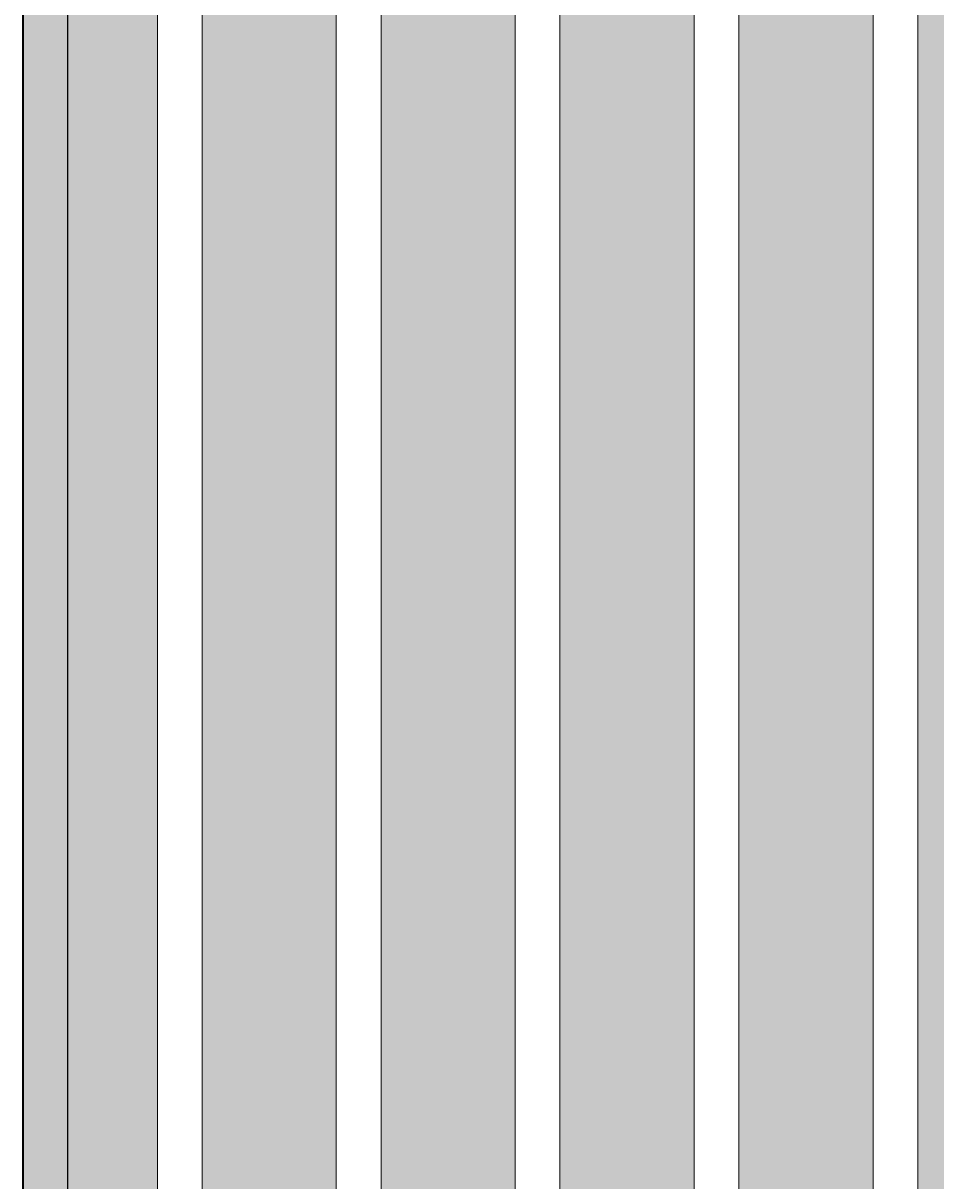
# Model space of a CAD drawing. Units: inches. Extents: x 4508 to 4723, y 847 to 1020.
# Tile 11 of 32: x 4550 to 4570, y 931 to 956. Entities that reach past the tile are written whole.
import ezdxf

# ---------------------------------------------------------------- set-up
doc = ezdxf.new("R2010")
doc.units = ezdxf.units.IN
for name, color, linetype, lineweight in [('A-ANNO-DIMS', 2, 'Continuous', 18), ('A-WALL', 7, 'Continuous', 35), ('A-WALL-FINS', 30, 'Continuous', 18), ('A-WALL-PATT', 254, 'Continuous', 13)]:
    doc.layers.add(name, color=color, linetype=linetype, lineweight=lineweight)
doc.styles.get("Standard").update_dxf_attribs({"font": 'arial.ttf'})
doc.dimstyles.get("Standard").update_dxf_attribs({"dimtxt": 0.18, "dimasz": 0.18, "dimexe": 0.18, "dimexo": 0.0625, "dimgap": 0.09, "dimtad": 0, "dimtih": 1, "dimtoh": 1, "dimdec": 4, "dimzin": 0, "dimdsep": 46, "dimtxsty": 'Standard', "dimcen": 0.09, "dimadec": 0, "dimazin": 0, "dimtfac": 1, "dimtdec": 4, "dimtofl": 0, "dimtmove": 0, "dimatfit": 3, "dimfxl": 1, "dimtolj": 1, "dimtzin": 0, "dimarcsym": 0})

# ---------------------------------------------------------------- blocks, each defined once
blk = doc.blocks.new('*D26')
at = {"layer": 'A-ANNO-DIMS', "color": 0, "lineweight": -2, "transparency": 16777216}
for p, q in [((4549.994, 904.809), (4549.994, 1002.877)), ((4550.994, 903.809), (4550.994, 1002.877)), ((4550.174, 1002.697), (4550.371, 1002.697)), ((4550.814, 1002.697), (4550.617, 1002.697))]:
    blk.add_line(p, q, dxfattribs=at)
at = {"layer": 'A-ANNO-DIMS', "color": 0, "lineweight": 9, "transparency": 16777216}
for points in [[(4550.174, 1002.727), (4550.174, 1002.667), (4549.994, 1002.697)], [(4550.814, 1002.727), (4550.814, 1002.667), (4550.994, 1002.697)]]:
    blk.add_solid(points, dxfattribs=at)
at = {"layer": 'Defpoints', "color": 0, "lineweight": 9, "transparency": 16777216}
for p in [(4550.994, 1002.697), (4549.994, 904.747), (4550.994, 903.747)]:
    blk.add_point(p, dxfattribs=at)
at = {"layer": 'A-ANNO-DIMS', "color": 0, "transparency": 16777216, "insert": (4550.494, 1002.697), "char_height": 0.18, "attachment_point": 5}
blk.add_mtext('\\A1;1', dxfattribs=at)
blk = doc.blocks.new('*D27')
at = {"layer": 'A-ANNO-DIMS', "color": 0, "lineweight": -2, "transparency": 16777216}
for p, q in [((4550.994, 903.809), (4550.994, 1002.877)), ((4577.494, 903.809), (4577.494, 1002.877)), ((4551.174, 1002.697), (4563.918, 1002.697)), ((4577.314, 1002.697), (4564.57, 1002.697))]:
    blk.add_line(p, q, dxfattribs=at)
at = {"layer": 'A-ANNO-DIMS', "color": 0, "lineweight": 9, "transparency": 16777216}
for points in [[(4551.174, 1002.727), (4551.174, 1002.667), (4550.994, 1002.697)], [(4577.314, 1002.727), (4577.314, 1002.667), (4577.494, 1002.697)]]:
    blk.add_solid(points, dxfattribs=at)
at = {"layer": 'Defpoints', "color": 0, "lineweight": 9, "transparency": 16777216}
for p in [(4577.494, 1002.697), (4550.994, 903.747), (4577.494, 903.747)]:
    blk.add_point(p, dxfattribs=at)
at = {"layer": 'A-ANNO-DIMS', "color": 0, "transparency": 16777216, "insert": (4564.244, 1002.697), "char_height": 0.18, "attachment_point": 5}
blk.add_mtext('\\A1;26.5', dxfattribs=at)

msp = doc.modelspace()

# ---------------------------------------------------------------- hatches: boundary and pattern name
at = {"layer": 'A-WALL-PATT', "transparency": 33554681}
h = msp.add_hatch(color=256, dxfattribs=at)
h.dxf.hatch_style = 1
h.paths.add_polyline_path([(4552.9938, 994.7469), (4549.9938, 994.7469), (4549.9938, 904.7469), (4552.9938, 904.7469)])
h.paths.add_polyline_path([(4556.9938, 994.7469), (4553.9938, 994.7469), (4553.9938, 904.7469), (4556.9938, 904.7469)])
h.paths.add_polyline_path([(4560.9938, 994.7469), (4557.9938, 994.7469), (4557.9938, 904.7469), (4560.9938, 904.7469)])
h.paths.add_polyline_path([(4564.9938, 994.7469), (4561.9938, 994.7469), (4561.9938, 904.7469), (4564.9938, 904.7469)])
h.paths.add_polyline_path([(4568.9938, 994.7469), (4565.9938, 994.7469), (4565.9938, 904.7469), (4568.9938, 904.7469)])
h.paths.add_polyline_path([(4572.9938, 994.7469), (4569.9938, 994.7469), (4569.9938, 904.7469), (4572.9938, 904.7469)])
h.paths.add_polyline_path([(4576.9938, 994.7469), (4573.9938, 994.7469), (4573.9938, 904.7469), (4576.9938, 904.7469)])
h.paths.add_polyline_path([(4580.9938, 994.7469), (4577.9938, 994.7469), (4577.9938, 904.7469), (4580.9938, 904.7469)])
h.paths.add_polyline_path([(4584.9938, 994.7469), (4581.9938, 994.7469), (4581.9938, 904.7469), (4584.9938, 904.7469)])

# ---------------------------------------------------------------- linework, layer by layer
at = {"layer": 'A-WALL'}
msp.add_line((4549.9938, 874.7469), (4549.9938, 994.7469), dxfattribs=at)
at = {"layer": 'A-WALL-FINS'}
for p, q in [((4552.9938, 904.7469), (4552.9938, 994.7469)), ((4553.9938, 904.7469), (4553.9938, 994.7469)), ((4556.9938, 904.7469), (4556.9938, 994.7469)), ((4557.9938, 904.7469), (4557.9938, 994.7469)), ((4560.9938, 904.7469), (4560.9938, 994.7469)), ((4561.9938, 904.7469), (4561.9938, 994.7469)), ((4564.9938, 904.7469), (4564.9938, 994.7469)), ((4565.9938, 904.7469), (4565.9938, 994.7469)), ((4568.9938, 904.7469), (4568.9938, 994.7469)), ((4569.9938, 904.7469), (4569.9938, 994.7469))]:
    msp.add_line(p, q, dxfattribs=at)

# ---------------------------------------------------------------- dimensions: what is measured, and where the dimension line sits
at = {"layer": 'A-ANNO-DIMS'}
for base, p1, p2, override, picture, middle in [((4550.9938, 1002.6969), (4549.9938, 904.7469), (4550.9938, 903.7469), {"dimdec": 0, "dimlfac": 1, "dimrnd": 0, "dimzin": 0, "dimdsep": 46, "dimlunit": 2}, '*D26', (4550.4938, 1002.6969)), ((4577.4938, 1002.6969), (4550.9938, 903.7469), (4577.4938, 903.7469), {"dimdec": 1, "dimlfac": 1, "dimrnd": 0, "dimzin": 0, "dimdsep": 46, "dimlunit": 2}, '*D27', (4564.2438, 1002.6969))]:
    dim = msp.add_linear_dim(base=base, p1=p1, p2=p2, dimstyle='Standard', override=override, dxfattribs=at)
    dim.commit()
    dim.dimension.update_dxf_attribs({"geometry": picture, "text_midpoint": middle})

doc.saveas('drawing.dxf')
